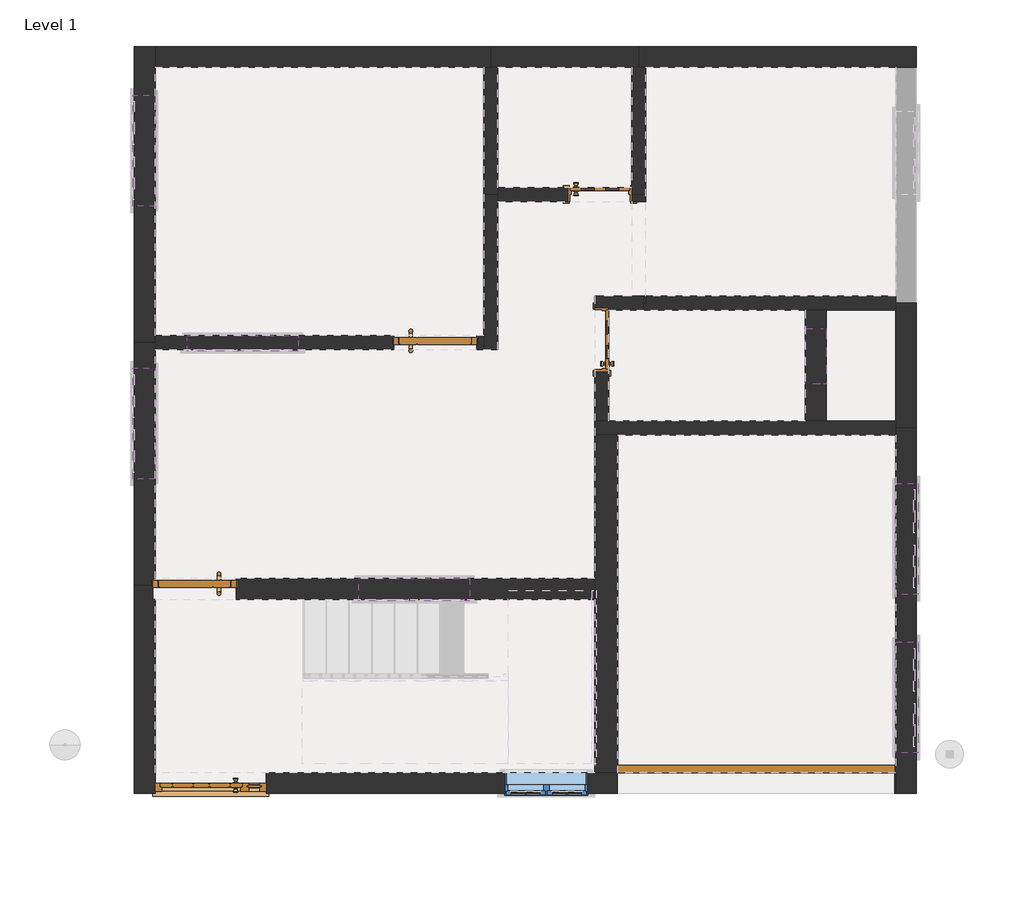
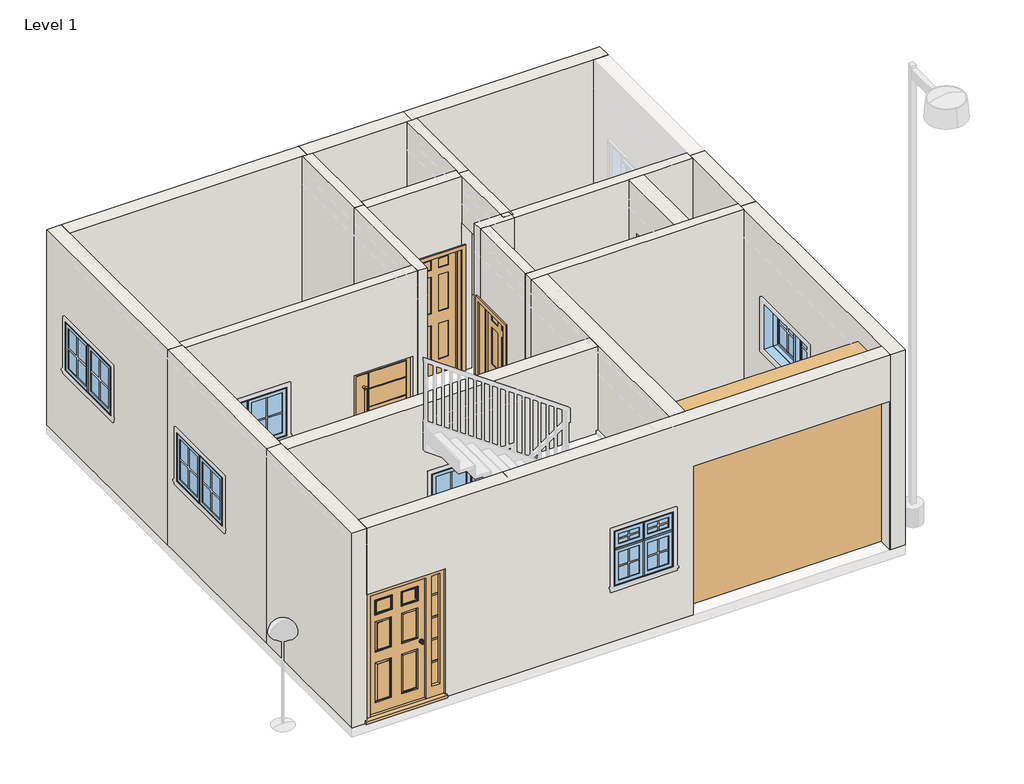
# One storey, part 1 of 3: 22 walls, 8 windows, 6 doors.
"""IFC4 building model written with IfcOpenShell, lengths in millimetres."""

from ifc_helpers import new_model, si_unit, frame, origin, place, context, project, spatial, polyline, outline, extrude, faceted_brep, transform, mapped, element, save
from components import door_3_ad1505b7, door_3_3562bf2b, extsgl_w_side_panel_4_ddded634, door_c4e61f94, door_c896847d, m_door_overhead_rolling_10_f67a646e, m_fixed_2_dd9f9b20, m_window_awning_double_horizontal_4_8afcb0b2, m_window_awning_double_horizontal_4_cab21571, m_window_casement_double_awning_double_3_6fa9dbfe

model = new_model("IFC4")

# Units and contexts
model_context = context("Model", 3, world=origin())
ifc_project = project(units=[si_unit("LENGTHUNIT", "METRE", prefix="MILLI")], contexts=[model_context])

# Site, building, storey
site = spatial("IfcSite", under=ifc_project)
building = spatial("IfcBuilding", under=site)
storey = spatial("IfcBuildingStorey", under=building, Name="Level 1", Elevation=0.0)

# Doors
placement = place(None, origin())
door_3_shape = door_3_ad1505b7(model_context)
element("IfcDoor", 1, ObjectType="3'", at=placement, inside=storey, context=model_context, shape_type="MappedRepresentation", body=[
    mapped(door_3_shape, transform((-8356.4282945, 391.3578397, 0.0), x_axis=(1.0, 0.0, 0.0), y_axis=(0.0, 1.0, 0.0), z_axis=(0.0, 0.0, 1.0))),
])
door_3_2_shape = door_3_3562bf2b(model_context)
element("IfcDoor", 2, ObjectType="3'", at=placement, inside=storey, context=model_context, shape_type="MappedRepresentation", body=[
    mapped(door_3_2_shape, transform((-10998.0282945, -2313.7421603, 0.0), x_axis=(-1.0, 0.0, 0.0), y_axis=(0.0, -1.0, 0.0), z_axis=(0.0, 0.0, 1.0))),
])
extsgl_w_side_panel_4_shape = extsgl_w_side_panel_4_ddded634(model_context)
element("IfcDoor", 3, ObjectType="ExtSgl w Side Panel : 4'", at=placement, inside=storey, context=model_context, shape_type="MappedRepresentation", body=[
    mapped(extsgl_w_side_panel_4_shape, transform((-11039.6282945, -4447.3421603, 0.0), x_axis=(-1.0, 0.0, 0.0), y_axis=(0.0, -1.0, 0.0), z_axis=(0.0, 0.0, 1.0))),
])
door_shape = door_c4e61f94(model_context)
element("IfcDoor", 4, ObjectType="M_Door-Interior-Single-6_Panel-Wood : 650 x 2000mm", at=placement, inside=storey, context=model_context, shape_type="MappedRepresentation", body=[
    mapped(door_shape, transform((-6547.4282945, 2020.1328397, 0.0), x_axis=(1.0, 0.0, 0.0), y_axis=(0.0, 1.0, 0.0), z_axis=(0.0, 0.0, 1.0))),
])
door_2_shape = door_c896847d(model_context)
element("IfcDoor", 5, ObjectType="M_Door-Interior-Single-6_Panel-Wood : 650 x 2000mm", at=placement, inside=storey, context=model_context, shape_type="MappedRepresentation", body=[
    mapped(door_2_shape, transform((-6524.4532945, 422.3578397, 0.0), x_axis=(0.0, 1.0, 0.0), y_axis=(-1.0, 0.0, 0.0), z_axis=(0.0, 0.0, 1.0))),
])
m_door_overhead_rolling_10_shape = m_door_overhead_rolling_10_f67a646e(model_context)
element("IfcDoor", 6, ObjectType="M_Door-Overhead-Rolling : 10'", at=placement, inside=storey, context=model_context, shape_type="MappedRepresentation", body=[
    mapped(m_door_overhead_rolling_10_shape, transform((-4834.0282945, -4447.3421603, 0.0289063), x_axis=(1.0, 0.0, 0.0), y_axis=(0.0, 1.0, 0.0), z_axis=(0.0, 0.0, 1.0))),
])

# Walls
element("IfcWall", 7, ObjectType="10\"", at=placement, inside=storey, context=model_context, shape_type="Brep", body=[
    faceted_brep([(-6603.8282945, -624.6421603, 0.0), (-6603.8282945, -2199.4421603, 0.0), (-6603.8282945, -2428.0421603, 0.0), (-6603.8282945, -4333.0421603, 0.0), (-6603.8282945, -4333.0421603, 3200.4), (-6603.8282945, -2428.0421603, 3200.4), (-6603.8282945, -2199.4421603, 3200.4), (-6603.8282945, -624.6421603, 3200.4), (-6349.8282945, -624.6421603, 0.0), (-6349.8282945, -624.6421603, 3200.4), (-6349.8282945, -4333.0421603, 3200.4), (-6349.8282945, -4333.0421603, 0.0)], [[[0, 1, 2, 3, 4, 5, 6, 7]], [[8, 9, 10, 11]], [[3, 2, 1, 0, 8, 11]], [[7, 6, 5, 4, 10, 9]], [[0, 7, 9, 8]], [[4, 3, 11, 10]]]),
])
element("IfcWall", 8, ObjectType="6\"", at=placement, inside=storey, context=model_context, shape_type="Brep", body=[
    faceted_brep([(-6197.4282945, 2016.9578397, 3200.4), (-6197.4282945, 2093.1578397, 3200.4), (-6197.4282945, 3413.9578397, 3200.4), (-6197.4282945, 3413.9578397, 0.0), (-6197.4282945, 2093.1578397, 0.0), (-6197.4282945, 2093.1578397, 2025.0), (-6197.4282945, 2016.9578397, 2025.0), (-6045.0282945, 2016.9578397, 0.0), (-6045.0282945, 3413.9578397, 0.0), (-6045.0282945, 3413.9578397, 3200.4), (-6045.0282945, 2016.9578397, 3200.4), (-6192.2282945, 2016.9578397, 0.0), (-6192.2282945, 2093.1578397, 0.0), (-6121.2282945, 3413.9578397, 0.0), (-6192.2282945, 2016.9578397, 2025.0), (-6121.2282945, 3413.9578397, 3200.4), (-6192.2282945, 2093.1578397, 2025.0)], [[[0, 1, 2, 3, 4, 5, 6]], [[7, 8, 9, 10]], [[8, 7, 11, 12, 4, 3, 13]], [[7, 10, 0, 6, 14, 11]], [[2, 1, 0, 10, 9, 15]], [[3, 2, 15, 9, 8, 13]], [[12, 16, 5, 4]], [[16, 12, 11, 14]], [[5, 16, 14, 6]]]),
])
element("IfcWall", 9, ObjectType="6\"", at=placement, inside=storey, context=model_context, shape_type="Brep", body=[
    faceted_brep([(-6070.4282945, 746.9578397, 0.0), (-6070.4282945, 746.9578397, 3200.4), (-6451.4282945, 746.9578397, 3200.4), (-6603.8282945, 746.9578397, 3200.4), (-6603.8282945, 746.9578397, 2025.0), (-6451.4282945, 746.9578397, 2025.0), (-6451.4282945, 746.9578397, 0.0), (-6070.4282945, 899.3578397, 0.0), (-6603.8282945, 899.3578397, 0.0), (-6603.8282945, 899.3578397, 3200.4), (-6070.4282945, 899.3578397, 3200.4), (-6451.4282945, 777.5578397, 0.0), (-6603.8282945, 777.5578397, 0.0), (-6603.8282945, 777.5578397, 2025.0), (-6451.4282945, 777.5578397, 2025.0)], [[[0, 1, 2, 3, 4, 5, 6]], [[7, 8, 9, 10]], [[8, 7, 0, 6, 11, 12]], [[1, 0, 7, 10]], [[3, 2, 1, 10, 9]], [[3, 9, 8, 12, 13, 4]], [[14, 11, 6, 5]], [[13, 14, 5, 4]], [[11, 14, 13, 12]]]),
])
element("IfcWall", 10, ObjectType="6\"", at=placement, inside=storey, context=model_context, shape_type="Brep", body=[
    faceted_brep([(-3301.8282945, -472.2421603, 0.0), (-4063.8282945, -472.2421603, 0.0), (-4292.4282945, -472.2421603, 0.0), (-6451.4282945, -472.2421603, 0.0), (-6603.8282945, -472.2421603, 0.0), (-6603.8282945, -472.2421603, 3200.4), (-6451.4282945, -472.2421603, 3200.4), (-4292.4282945, -472.2421603, 3200.4), (-4063.8282945, -472.2421603, 3200.4), (-3301.8282945, -472.2421603, 3200.4), (-3301.8282945, -624.6421603, 0.0), (-3301.8282945, -624.6421603, 3200.4), (-6349.8282945, -624.6421603, 3200.4), (-6603.8282945, -624.6421603, 3200.4), (-6603.8282945, -624.6421603, 0.0), (-6349.8282945, -624.6421603, 0.0), (-3301.8282945, -548.4421603, 0.0), (-3301.8282945, -548.4421603, 3200.4)], [[[0, 1, 2, 3, 4, 5, 6, 7, 8, 9]], [[10, 11, 12, 13, 14, 15]], [[4, 3, 2, 1, 0, 16, 10, 15, 14]], [[9, 8, 7, 6, 5, 13, 12, 11, 17]], [[0, 9, 17, 11, 10, 16]], [[5, 4, 14, 13]]]),
])
element("IfcWall", 11, ObjectType="6\"", at=placement, inside=storey, context=model_context, shape_type="Brep", body=[
    faceted_brep([(-7823.0282945, 3413.9578397, 0.0), (-7823.0282945, 2016.9578397, 0.0), (-7823.0282945, 2016.9578397, 3200.4), (-7823.0282945, 3413.9578397, 3200.4), (-7670.6282945, 3413.9578397, 0.0), (-7670.6282945, 3413.9578397, 3200.4), (-7670.6282945, 2093.1578397, 3200.4), (-7670.6282945, 2016.9578397, 3200.4), (-7670.6282945, 2016.9578397, 0.0), (-7670.6282945, 2093.1578397, 0.0), (-7746.8282945, 3413.9578397, 0.0), (-7746.8282945, 3413.9578397, 3200.4)], [[[0, 1, 2, 3]], [[4, 5, 6, 7, 8, 9]], [[1, 0, 10, 4, 9, 8]], [[2, 1, 8, 7]], [[3, 2, 7, 6, 5, 11]], [[0, 3, 11, 5, 4, 10]]]),
])
element("IfcWall", 12, ObjectType="6\"", at=placement, inside=storey, context=model_context, shape_type="Brep", body=[
    faceted_brep([(-7823.0282945, 315.1578397, 3200.4), (-11429.8282945, 315.1578397, 3200.4), (-11429.8282945, 315.1578397, 0.0), (-8813.6282945, 315.1578397, 0.0), (-8813.6282945, 315.1578397, 1828.8), (-7899.2282945, 315.1578397, 1828.8), (-7899.2282945, 315.1578397, 0.0), (-7823.0282945, 315.1578397, 0.0), (-11078.1970445, 315.1578397, 2019.2), (-9858.9970445, 315.1578397, 2019.2), (-9858.9970445, 315.1578397, 1219.2), (-11078.1970445, 315.1578397, 1219.2), (-11429.8282945, 467.5578397, 3200.4), (-7823.0282945, 467.5578397, 3200.4), (-7823.0282945, 467.5578397, 0.0), (-7899.2282945, 467.5578397, 0.0), (-7899.2282945, 467.5578397, 1828.8), (-8813.6282945, 467.5578397, 1828.8), (-8813.6282945, 467.5578397, 0.0), (-11429.8282945, 467.5578397, 0.0), (-11078.1970445, 467.5578397, 2019.2), (-11078.1970445, 467.5578397, 1219.2), (-9858.9970445, 467.5578397, 1219.2), (-9858.9970445, 467.5578397, 2019.2), (-11429.8282945, 391.3578397, 0.0), (-8813.6282945, 447.5578397, 0.0), (-8828.6282945, 447.5578397, 0.0), (-8828.6282945, 370.5578397, 0.0), (-8813.6282945, 370.5578397, 0.0), (-7899.2282945, 370.5578397, 0.0), (-7884.2282945, 370.5578397, 0.0), (-7884.2282945, 447.5578397, 0.0), (-7899.2282945, 447.5578397, 0.0), (-11429.8282945, 391.3578397, 3200.4), (-7899.2282945, 447.5578397, 1828.8), (-8813.6282945, 447.5578397, 1828.8), (-8813.6282945, 370.5578397, 1828.8), (-7899.2282945, 370.5578397, 1828.8), (-8828.6282945, 447.5578397, 1843.8), (-7884.2282945, 447.5578397, 1843.8), (-7884.2282945, 370.5578397, 1843.8), (-8828.6282945, 370.5578397, 1843.8)], [[[0, 1, 2, 3, 4, 5, 6, 7], [8, 9, 10, 11]], [[12, 13, 14, 15, 16, 17, 18, 19], [20, 21, 22, 23]], [[2, 24, 19, 18, 25, 26, 27, 28, 3]], [[14, 7, 6, 29, 30, 31, 32, 15]], [[1, 0, 13, 12, 33]], [[0, 7, 14, 13]], [[2, 1, 33, 12, 19, 24]], [[16, 34, 35, 17]], [[4, 36, 37, 5]], [[34, 16, 15, 32]], [[5, 37, 29, 6]], [[17, 35, 25, 18]], [[36, 4, 3, 28]], [[38, 39, 40, 41]], [[40, 39, 31, 30]], [[37, 36, 28, 27, 41, 40, 30, 29]], [[38, 41, 27, 26]], [[35, 34, 32, 31, 39, 38, 26, 25]], [[21, 20, 8, 11]], [[22, 21, 11, 10]], [[23, 22, 10, 9]], [[20, 23, 9, 8]]]),
])
element("IfcWall", 13, ObjectType="6\"", at=placement, inside=storey, context=model_context, shape_type="Brep", body=[
    faceted_brep([(-6197.4282945, 1940.7578397, 3200.4), (-7670.6282945, 1940.7578397, 3200.4), (-7670.6282945, 1940.7578397, 0.0), (-6902.6282945, 1940.7578397, 0.0), (-6902.6282945, 1940.7578397, 2025.0), (-6197.4282945, 1940.7578397, 2025.0), (-7670.6282945, 2093.1578397, 3200.4), (-6197.4282945, 2093.1578397, 3200.4), (-6197.4282945, 2093.1578397, 2025.0), (-6902.6282945, 2093.1578397, 2025.0), (-6902.6282945, 2093.1578397, 0.0), (-7670.6282945, 2093.1578397, 0.0), (-7670.6282945, 2016.9578397, 0.0), (-6197.4282945, 2016.9578397, 3200.4), (-7670.6282945, 2016.9578397, 3200.4), (-6197.4282945, 2016.9578397, 2025.0)], [[[0, 1, 2, 3, 4, 5]], [[6, 7, 8, 9, 10, 11]], [[2, 12, 11, 10, 3]], [[1, 0, 13, 7, 6, 14]], [[7, 13, 0, 5, 15, 8]], [[2, 1, 14, 6, 11, 12]], [[4, 9, 8, 15, 5]], [[9, 4, 3, 10]]]),
])
element("IfcWall", 14, ObjectType="6\"", at=placement, inside=storey, context=model_context, shape_type="SweptSolid", body=[
    extrude(outline(polyline([(-472.2421603, 3200.4), (746.9578397, 3200.4), (746.9578397, 2025.0), (67.1578397, 2025.0), (67.1578397, 0.0), (-472.2421603, 0.0), (-472.2421603, 3200.4)])), frame((-6603.8282945, 0.0, 0.0), z_axis=(1.0, 0.0, 0.0), x_axis=(0.0, 1.0, 0.0)), (0.0, 0.0, 1.0), 152.4),
])
element("IfcWall", 15, ObjectType="6\"", at=placement, inside=storey, context=model_context, shape_type="Brep", body=[
    faceted_brep([(-7823.0282945, 2016.9578397, 0.0), (-7823.0282945, 467.5578397, 0.0), (-7823.0282945, 315.1578397, 0.0), (-7823.0282945, 315.1578397, 3200.4), (-7823.0282945, 467.5578397, 3200.4), (-7823.0282945, 2016.9578397, 3200.4), (-7670.6282945, 2016.9578397, 0.0), (-7670.6282945, 2016.9578397, 3200.4), (-7670.6282945, 1940.7578397, 3200.4), (-7670.6282945, 315.1578397, 3200.4), (-7670.6282945, 315.1578397, 0.0), (-7670.6282945, 1940.7578397, 0.0)], [[[0, 1, 2, 3, 4, 5]], [[6, 7, 8, 9, 10, 11]], [[2, 1, 0, 6, 11, 10]], [[5, 4, 3, 9, 8, 7]], [[0, 5, 7, 6]], [[3, 2, 10, 9]]]),
])
element("IfcWall", 16, ObjectType="6\"", at=placement, inside=storey, context=model_context, shape_type="Brep", body=[
    faceted_brep([(-6197.4282945, 823.1578397, 0.0), (-6197.4282945, 823.1578397, 3200.4), (-6197.4282945, 1940.7578397, 3200.4), (-6197.4282945, 2016.9578397, 3200.4), (-6197.4282945, 2016.9578397, 2025.0), (-6197.4282945, 1940.7578397, 2025.0), (-6197.4282945, 1940.7578397, 0.0), (-6197.4282945, 1939.2741832, 0.0), (-6197.4282945, 1939.2741832, 2438.4), (-6197.4282945, 896.0499365, 2438.4), (-6197.4282945, 896.0499365, 0.0), (-6045.0282945, 823.1578397, 3200.4), (-6045.0282945, 823.1578397, 0.0), (-6045.0282945, 896.0499365, 0.0), (-6045.0282945, 896.0499365, 2438.4), (-6045.0282945, 1939.2741832, 2438.4), (-6045.0282945, 1939.2741832, 0.0), (-6045.0282945, 2016.9578397, 0.0), (-6045.0282945, 2016.9578397, 3200.4), (-6192.2282945, 1940.7578397, 0.0), (-6192.2282945, 2016.9578397, 0.0), (-6192.2282945, 2016.9578397, 2025.0), (-6192.2282945, 1940.7578397, 2025.0)], [[[0, 1, 2, 3, 4, 5, 6, 7, 8, 9, 10]], [[11, 12, 13, 14, 15, 16, 17, 18]], [[12, 0, 10, 13]], [[17, 16, 7, 6, 19, 20]], [[1, 0, 12, 11]], [[3, 2, 1, 11, 18]], [[18, 17, 20, 21, 4, 3]], [[8, 15, 14, 9]], [[15, 8, 7, 16]], [[9, 14, 13, 10]], [[22, 19, 6, 5]], [[19, 22, 21, 20]], [[22, 5, 4, 21]]]),
])
element("IfcWall", 17, ObjectType="6\"", at=placement, inside=storey, context=model_context, shape_type="Brep", body=[
    faceted_brep([(-6070.4282945, 746.9578397, 0.0), (-4292.4282945, 746.9578397, 0.0), (-4063.8282945, 746.9578397, 0.0), (-3301.8282945, 746.9578397, 0.0), (-3301.8282945, 746.9578397, 3200.4), (-4063.8282945, 746.9578397, 3200.4), (-4292.4282945, 746.9578397, 3200.4), (-6070.4282945, 746.9578397, 3200.4), (-6070.4282945, 899.3578397, 0.0), (-6070.4282945, 899.3578397, 3200.4), (-3301.8282945, 899.3578397, 3200.4), (-3301.8282945, 899.3578397, 0.0), (-3301.8282945, 823.1578397, 0.0), (-3301.8282945, 823.1578397, 3200.4)], [[[0, 1, 2, 3, 4, 5, 6, 7]], [[8, 9, 10, 11]], [[3, 2, 1, 0, 8, 11, 12]], [[7, 6, 5, 4, 13, 10, 9]], [[0, 7, 9, 8]], [[4, 3, 12, 11, 10, 13]]]),
])
element("IfcWall", 18, ObjectType="9\"", at=placement, inside=storey, context=model_context, shape_type="Brep", body=[
    faceted_brep([(-11658.4282945, 3642.5578397, 0.0), (-11658.4282945, 391.3578397, 0.0), (-11658.4282945, 391.3578397, 3200.4), (-11658.4282945, 3642.5578397, 3200.4), (-11658.4282945, 3109.1578397, 2019.2), (-11658.4282945, 1889.9578397, 2019.2), (-11658.4282945, 1889.9578397, 1219.2), (-11658.4282945, 3109.1578397, 1219.2), (-11429.8282945, 3642.5578397, 0.0), (-11429.8282945, 3642.5578397, 3200.4), (-11429.8282945, 3413.9578397, 3200.4), (-11429.8282945, 467.5578397, 3200.4), (-11429.8282945, 391.3578397, 3200.4), (-11429.8282945, 391.3578397, 0.0), (-11429.8282945, 467.5578397, 0.0), (-11429.8282945, 3413.9578397, 0.0), (-11429.8282945, 3109.1578397, 2019.2), (-11429.8282945, 3109.1578397, 1219.2), (-11429.8282945, 1889.9578397, 1219.2), (-11429.8282945, 1889.9578397, 2019.2)], [[[0, 1, 2, 3], [4, 5, 6, 7]], [[8, 9, 10, 11, 12, 13, 14, 15], [16, 17, 18, 19]], [[1, 0, 8, 15, 14, 13]], [[2, 1, 13, 12]], [[3, 2, 12, 11, 10, 9]], [[0, 3, 9, 8]], [[17, 16, 4, 7]], [[18, 17, 7, 6]], [[19, 18, 6, 5]], [[16, 19, 5, 4]]]),
])
element("IfcWall", 19, ObjectType="9\"", at=placement, inside=storey, context=model_context, shape_type="Brep", body=[
    faceted_brep([(-11429.8282945, 3413.9578397, 0.0), (-7823.0282945, 3413.9578397, 0.0), (-7746.8282945, 3413.9578397, 0.0), (-7746.8282945, 3413.9578397, 3200.4), (-7823.0282945, 3413.9578397, 3200.4), (-11429.8282945, 3413.9578397, 3200.4), (-11429.8282945, 3642.5578397, 0.0), (-11429.8282945, 3642.5578397, 3200.4), (-7746.8282945, 3642.5578397, 3200.4), (-7746.8282945, 3642.5578397, 0.0)], [[[0, 1, 2, 3, 4, 5]], [[6, 7, 8, 9]], [[2, 1, 0, 6, 9]], [[3, 2, 9, 8]], [[5, 4, 3, 8, 7]], [[0, 5, 7, 6]]]),
])
element("IfcWall", 20, ObjectType="9\"", at=placement, inside=storey, context=model_context, shape_type="Brep", body=[
    faceted_brep([(-11429.8282945, -4333.0421603, 3200.4), (-6603.8282945, -4333.0421603, 3200.4), (-6349.8282945, -4333.0421603, 3200.4), (-3301.8282945, -4333.0421603, 3200.4), (-3301.8282945, -4333.0421603, 0.0), (-3310.0282945, -4333.0421603, 0.0), (-3310.0282945, -4333.0421603, 2438.4289062), (-6358.0282945, -4333.0421603, 2438.4289062), (-6358.0282945, -4333.0421603, 0.0), (-6603.8282945, -4333.0421603, 0.0), (-10210.6282945, -4333.0421603, 0.0), (-10210.6282945, -4333.0421603, 2110.0), (-11429.8282945, -4333.0421603, 2110.0), (-7594.4282945, -4333.0421603, 1814.4), (-7594.4282945, -4333.0421603, 914.4), (-6680.0282945, -4333.0421603, 914.4), (-6680.0282945, -4333.0421603, 1814.4), (-3301.8282945, -4561.6421603, 3200.4), (-11429.8282945, -4561.6421603, 3200.4), (-11429.8282945, -4561.6421603, 2110.0), (-10210.6282945, -4561.6421603, 2110.0), (-10210.6282945, -4561.6421603, 0.0), (-6358.0282945, -4561.6421603, 0.0), (-6358.0282945, -4561.6421603, 2438.4289062), (-3310.0282945, -4561.6421603, 2438.4289062), (-3310.0282945, -4561.6421603, 0.0), (-3301.8282945, -4561.6421603, 0.0), (-7594.4282945, -4561.6421603, 1814.4), (-6680.0282945, -4561.6421603, 1814.4), (-6680.0282945, -4561.6421603, 914.4), (-7594.4282945, -4561.6421603, 914.4)], [[[0, 1, 2, 3, 4, 5, 6, 7, 8, 9, 10, 11, 12], [13, 14, 15, 16]], [[17, 18, 19, 20, 21, 22, 23, 24, 25, 26], [27, 28, 29, 30]], [[4, 26, 25, 5]], [[8, 22, 21, 10, 9]], [[3, 2, 1, 0, 18, 17]], [[18, 0, 12, 19]], [[4, 3, 17, 26]], [[6, 5, 25, 24]], [[7, 6, 24, 23]], [[8, 7, 23, 22]], [[20, 11, 10, 21]], [[11, 20, 19, 12]], [[14, 13, 27, 30]], [[15, 14, 30, 29]], [[16, 15, 29, 28]], [[13, 16, 28, 27]]]),
])
element("IfcWall", 21, ObjectType="9\"", at=placement, inside=storey, context=model_context, shape_type="Brep", body=[
    faceted_brep([(-11429.8282945, -2199.4421603, 3200.4), (-6603.8282945, -2199.4421603, 3200.4), (-6603.8282945, -2199.4421603, 0.0), (-10540.8282945, -2199.4421603, 0.0), (-10540.8282945, -2199.4421603, 1828.8), (-11429.8282945, -2199.4421603, 1828.8), (-9194.6282945, -2199.4421603, 2019.2), (-9194.6282945, -2199.4421603, 1219.2), (-7975.4282945, -2199.4421603, 1219.2), (-7975.4282945, -2199.4421603, 2019.2), (-6603.8282945, -2428.0421603, 3200.4), (-11429.8282945, -2428.0421603, 3200.4), (-11429.8282945, -2428.0421603, 1828.8), (-10540.8282945, -2428.0421603, 1828.8), (-10540.8282945, -2428.0421603, 0.0), (-6603.8282945, -2428.0421603, 0.0), (-9194.6282945, -2428.0421603, 2019.2), (-7975.4282945, -2428.0421603, 2019.2), (-7975.4282945, -2428.0421603, 1219.2), (-9194.6282945, -2428.0421603, 1219.2), (-10540.8282945, -2296.4421603, 0.0), (-10525.8282945, -2296.4421603, 0.0), (-10525.8282945, -2219.4421603, 0.0), (-10540.8282945, -2219.4421603, 0.0), (-11429.8282945, -2275.6421603, 3200.4), (-11429.8282945, -2219.4421603, 1828.8), (-11429.8282945, -2219.4421603, 1843.8), (-11429.8282945, -2296.4421603, 1843.8), (-11429.8282945, -2296.4421603, 1828.8), (-10540.8282945, -2219.4421603, 1828.8), (-10540.8282945, -2296.4421603, 1828.8), (-10525.8282945, -2219.4421603, 1843.8), (-10525.8282945, -2296.4421603, 1843.8)], [[[0, 1, 2, 3, 4, 5], [6, 7, 8, 9]], [[10, 11, 12, 13, 14, 15], [16, 17, 18, 19]], [[2, 15, 14, 20, 21, 22, 23, 3]], [[1, 0, 24, 11, 10]], [[11, 24, 0, 5, 25, 26, 27, 28, 12]], [[2, 1, 10, 15]], [[4, 29, 25, 5]], [[30, 13, 12, 28]], [[29, 4, 3, 23]], [[13, 30, 20, 14]], [[31, 32, 27, 26]], [[20, 30, 28, 27, 32, 21]], [[32, 31, 22, 21]], [[29, 23, 22, 31, 26, 25]], [[7, 6, 16, 19]], [[8, 7, 19, 18]], [[9, 8, 18, 17]], [[6, 9, 17, 16]]]),
])
element("IfcWall", 22, ObjectType="9\"", at=placement, inside=storey, context=model_context, shape_type="SweptSolid", body=[
    extrude(outline(polyline([(746.9578397, 0.0), (-472.2421603, 0.0), (-472.2421603, 3200.4), (746.9578397, 3200.4), (746.9578397, 0.0)]), holes=[polyline([(543.7578397, 2133.6), (543.7578397, 2438.4), (-65.8421603, 2438.4), (-65.8421603, 2133.6), (543.7578397, 2133.6)])]), frame((-4292.4282945, 0.0, 0.0), z_axis=(1.0, 0.0, 0.0), x_axis=(0.0, 1.0, 0.0)), (0.0, 0.0, 1.0), 228.6),
])
element("IfcWall", 23, ObjectType="9\"", at=placement, inside=storey, context=model_context, shape_type="Brep", body=[
    faceted_brep([(-11658.4282945, 391.3578397, 0.0), (-11658.4282945, -2275.6421603, 0.0), (-11658.4282945, -2275.6421603, 3200.4), (-11658.4282945, 391.3578397, 3200.4), (-11658.4282945, 111.9578397, 2019.2), (-11658.4282945, -1107.2421603, 2019.2), (-11658.4282945, -1107.2421603, 1219.2), (-11658.4282945, 111.9578397, 1219.2), (-11429.8282945, 391.3578397, 3200.4), (-11429.8282945, 315.1578397, 3200.4), (-11429.8282945, -2275.6421603, 3200.4), (-11429.8282945, -2275.6421603, 1843.8), (-11429.8282945, -2219.4421603, 1843.8), (-11429.8282945, -2219.4421603, 1828.8), (-11429.8282945, -2199.4421603, 1828.8), (-11429.8282945, -2199.4421603, 0.0), (-11429.8282945, 315.1578397, 0.0), (-11429.8282945, 391.3578397, 0.0), (-11429.8282945, 111.9578397, 2019.2), (-11429.8282945, 111.9578397, 1219.2), (-11429.8282945, -1107.2421603, 1219.2), (-11429.8282945, -1107.2421603, 2019.2), (-11455.2282945, -2199.4421603, 0.0), (-11455.2282945, -2219.4421603, 0.0), (-11470.2282945, -2219.4421603, 0.0), (-11470.2282945, -2275.6421603, 0.0), (-11470.2282945, -2275.6421603, 1843.8), (-11455.2282945, -2199.4421603, 1828.8), (-11455.2282945, -2219.4421603, 1828.8), (-11470.2282945, -2219.4421603, 1843.8)], [[[0, 1, 2, 3], [4, 5, 6, 7]], [[8, 9, 10, 11, 12, 13, 14, 15, 16, 17], [18, 19, 20, 21]], [[1, 0, 17, 16, 15, 22, 23, 24, 25]], [[2, 1, 25, 26, 11, 10]], [[3, 2, 10, 9, 8]], [[0, 3, 8, 17]], [[18, 21, 5, 4]], [[21, 20, 6, 5]], [[20, 19, 7, 6]], [[19, 18, 4, 7]], [[27, 22, 15, 14]], [[28, 27, 14, 13]], [[22, 27, 28, 23]], [[26, 29, 12, 11]], [[24, 29, 26, 25]], [[23, 28, 13, 12, 29, 24]]]),
])
element("IfcWall", 24, ObjectType="9\"", at=placement, inside=storey, context=model_context, shape_type="Brep", body=[
    faceted_brep([(-7746.8282945, 3413.9578397, 0.0), (-7670.6282945, 3413.9578397, 0.0), (-6197.4282945, 3413.9578397, 0.0), (-6121.2282945, 3413.9578397, 0.0), (-6121.2282945, 3413.9578397, 3200.4), (-6197.4282945, 3413.9578397, 3200.4), (-7670.6282945, 3413.9578397, 3200.4), (-7746.8282945, 3413.9578397, 3200.4), (-7746.8282945, 3642.5578397, 0.0), (-7746.8282945, 3642.5578397, 3200.4), (-6121.2282945, 3642.5578397, 3200.4), (-6121.2282945, 3642.5578397, 0.0)], [[[0, 1, 2, 3, 4, 5, 6, 7]], [[8, 9, 10, 11]], [[3, 2, 1, 0, 8, 11]], [[4, 3, 11, 10]], [[7, 6, 5, 4, 10, 9]], [[0, 7, 9, 8]]]),
])
element("IfcWall", 25, ObjectType="9\"", at=placement, inside=storey, context=model_context, shape_type="Brep", body=[
    faceted_brep([(-6121.2282945, 3413.9578397, 0.0), (-6045.0282945, 3413.9578397, 0.0), (-3301.8282945, 3413.9578397, 0.0), (-3073.2282945, 3413.9578397, 0.0), (-3073.2282945, 3413.9578397, 3200.4), (-3301.8282945, 3413.9578397, 3200.4), (-6045.0282945, 3413.9578397, 3200.4), (-6121.2282945, 3413.9578397, 3200.4), (-6121.2282945, 3642.5578397, 0.0), (-6121.2282945, 3642.5578397, 3200.4), (-3073.2282945, 3642.5578397, 3200.4), (-3073.2282945, 3642.5578397, 0.0)], [[[0, 1, 2, 3, 4, 5, 6, 7]], [[8, 9, 10, 11]], [[3, 2, 1, 0, 8, 11]], [[7, 6, 5, 4, 10, 9]], [[0, 7, 9, 8]], [[4, 3, 11, 10]]]),
])
element("IfcWall", 26, ObjectType="9\"", at=placement, inside=storey, context=model_context, shape_type="Brep", body=[
    faceted_brep([(-3301.8282945, 823.1578397, 0.0), (-3301.8282945, 746.9578397, 0.0), (-3301.8282945, -472.2421603, 0.0), (-3301.8282945, -548.4421603, 0.0), (-3301.8282945, -548.4421603, 3200.4), (-3301.8282945, -472.2421603, 3200.4), (-3301.8282945, 746.9578397, 3200.4), (-3301.8282945, 823.1578397, 3200.4), (-3073.2282945, 823.1578397, 0.0), (-3073.2282945, 823.1578397, 3200.4), (-3073.2282945, -548.4421603, 3200.4), (-3073.2282945, -548.4421603, 0.0)], [[[0, 1, 2, 3, 4, 5, 6, 7]], [[8, 9, 10, 11]], [[3, 2, 1, 0, 8, 11]], [[4, 3, 11, 10]], [[7, 6, 5, 4, 10, 9]], [[0, 7, 9, 8]]]),
])
element("IfcWall", 27, ObjectType="9\"", at=placement, inside=storey, context=model_context, shape_type="Brep", body=[
    faceted_brep([(-3301.8282945, -548.4421603, 0.0), (-3301.8282945, -624.6421603, 0.0), (-3301.8282945, -4333.0421603, 0.0), (-3301.8282945, -4561.6421603, 0.0), (-3301.8282945, -4561.6421603, 3200.4), (-3301.8282945, -4333.0421603, 3200.4), (-3301.8282945, -624.6421603, 3200.4), (-3301.8282945, -548.4421603, 3200.4), (-3301.8282945, -4117.1421603, 2019.2), (-3301.8282945, -4117.1421603, 1219.2), (-3301.8282945, -2897.9421603, 1219.2), (-3301.8282945, -2897.9421603, 2019.2), (-3301.8282945, -2374.4640353, 2019.2), (-3301.8282945, -2374.4640353, 1219.2), (-3301.8282945, -1155.2640353, 1219.2), (-3301.8282945, -1155.2640353, 2019.2), (-3073.2282945, -548.4421603, 0.0), (-3073.2282945, -548.4421603, 3200.4), (-3073.2282945, -4561.6421603, 3200.4), (-3073.2282945, -4561.6421603, 0.0), (-3073.2282945, -4117.1421603, 2019.2), (-3073.2282945, -2897.9421603, 2019.2), (-3073.2282945, -2897.9421603, 1219.2), (-3073.2282945, -4117.1421603, 1219.2), (-3073.2282945, -2374.4640353, 2019.2), (-3073.2282945, -1155.2640353, 2019.2), (-3073.2282945, -1155.2640353, 1219.2), (-3073.2282945, -2374.4640353, 1219.2)], [[[0, 1, 2, 3, 4, 5, 6, 7], [8, 9, 10, 11], [12, 13, 14, 15]], [[16, 17, 18, 19], [20, 21, 22, 23], [24, 25, 26, 27]], [[3, 2, 1, 0, 16, 19]], [[7, 6, 5, 4, 18, 17]], [[0, 7, 17, 16]], [[4, 3, 19, 18]], [[8, 11, 21, 20]], [[11, 10, 22, 21]], [[10, 9, 23, 22]], [[9, 8, 20, 23]], [[12, 15, 25, 24]], [[15, 14, 26, 25]], [[14, 13, 27, 26]], [[13, 12, 24, 27]]]),
])
element("IfcWall", 28, ObjectType="9\"", at=placement, inside=storey, context=model_context, shape_type="Brep", body=[
    faceted_brep([(-11658.4282945, -2275.6421603, 0.0), (-11658.4282945, -4561.6421603, 0.0), (-11658.4282945, -4561.6421603, 3200.4), (-11658.4282945, -2275.6421603, 3200.4), (-11429.8282945, -2275.6421603, 3200.4), (-11429.8282945, -2428.0421603, 3200.4), (-11429.8282945, -4333.0421603, 3200.4), (-11429.8282945, -4561.6421603, 3200.4), (-11429.8282945, -4561.6421603, 2110.0), (-11429.8282945, -4561.6421603, 0.0), (-11429.8282945, -2428.0421603, 0.0), (-11429.8282945, -2428.0421603, 1828.8), (-11429.8282945, -2296.4421603, 1828.8), (-11429.8282945, -2296.4421603, 1843.8), (-11429.8282945, -2275.6421603, 1843.8), (-11470.2282945, -2275.6421603, 0.0), (-11470.2282945, -2296.4421603, 0.0), (-11455.2282945, -2296.4421603, 0.0), (-11455.2282945, -2428.0421603, 0.0), (-11470.2282945, -2275.6421603, 1843.8), (-11455.2282945, -2428.0421603, 1828.8), (-11455.2282945, -2296.4421603, 1828.8), (-11470.2282945, -2296.4421603, 1843.8)], [[[0, 1, 2, 3]], [[4, 5, 6, 7, 8, 9, 10, 11, 12, 13, 14]], [[1, 0, 15, 16, 17, 18, 10, 9]], [[3, 2, 7, 6, 5, 4]], [[0, 3, 4, 14, 19, 15]], [[2, 1, 9, 8, 7]], [[18, 20, 11, 10]], [[20, 21, 12, 11]], [[20, 18, 17, 21]], [[13, 22, 19, 14]], [[22, 16, 15, 19]], [[21, 17, 16, 22, 13, 12]]]),
])

# Windows
m_fixed_2_shape = m_fixed_2_dd9f9b20(model_context)
element("IfcWindow", 29, ObjectType="M_Fixed : 2'", at=placement, inside=storey, context=model_context, shape_type="MappedRepresentation", body=[
    mapped(m_fixed_2_shape, transform((-4191.1282945, 238.9578397, 1218.6), x_axis=(0.0, -1.0, 0.0), y_axis=(1.0, 0.0, 0.0), z_axis=(0.0, 0.0, 1.0))),
])
m_window_awning_double_horizontal_4_shape = m_window_awning_double_horizontal_4_8afcb0b2(model_context)
element("IfcWindow", 30, ObjectType="M_Window-Awning-Double-Horizontal : 4'", at=placement, inside=storey, context=model_context, shape_type="MappedRepresentation", body=[
    mapped(m_window_awning_double_horizontal_4_shape, transform((-8585.0282945, -2313.7421603, 319.2), x_axis=(-1.0, 0.0, 0.0), y_axis=(0.0, -1.0, 0.0), z_axis=(0.0, 0.0, 1.0))),
])
element("IfcWindow", 31, ObjectType="M_Window-Awning-Double-Horizontal : 4'", at=placement, inside=storey, context=model_context, shape_type="MappedRepresentation", body=[
    mapped(m_window_awning_double_horizontal_4_shape, transform((-3187.5282945, -3507.5421603, 319.2), x_axis=(0.0, -1.0, 0.0), y_axis=(1.0, 0.0, 0.0), z_axis=(0.0, 0.0, 1.0))),
])
element("IfcWindow", 32, ObjectType="M_Window-Awning-Double-Horizontal : 4'", at=placement, inside=storey, context=model_context, shape_type="MappedRepresentation", body=[
    mapped(m_window_awning_double_horizontal_4_shape, transform((-3187.5282945, -1764.8640353, 319.2), x_axis=(0.0, -1.0, 0.0), y_axis=(1.0, 0.0, 0.0), z_axis=(0.0, 0.0, 1.0))),
])
element("IfcWindow", 33, ObjectType="M_Window-Awning-Double-Horizontal : 4'", at=placement, inside=storey, context=model_context, shape_type="MappedRepresentation", body=[
    mapped(m_window_awning_double_horizontal_4_shape, transform((-11544.1282945, 2499.5578397, 319.2), x_axis=(0.0, 1.0, 0.0), y_axis=(-1.0, 0.0, 0.0), z_axis=(0.0, 0.0, 1.0))),
])
element("IfcWindow", 34, ObjectType="M_Window-Awning-Double-Horizontal : 4'", at=placement, inside=storey, context=model_context, shape_type="MappedRepresentation", body=[
    mapped(m_window_awning_double_horizontal_4_shape, transform((-11544.1282945, -497.6421603, 319.2), x_axis=(0.0, 1.0, 0.0), y_axis=(-1.0, 0.0, 0.0), z_axis=(0.0, 0.0, 1.0))),
])
m_window_awning_double_horizontal_4_2_shape = m_window_awning_double_horizontal_4_cab21571(model_context)
element("IfcWindow", 35, ObjectType="M_Window-Awning-Double-Horizontal : 4'", at=placement, inside=storey, context=model_context, shape_type="MappedRepresentation", body=[
    mapped(m_window_awning_double_horizontal_4_2_shape, transform((-10468.5970445, 391.3578397, 319.2), x_axis=(-1.0, 0.0, 0.0), y_axis=(0.0, -1.0, 0.0), z_axis=(0.0, 0.0, 1.0))),
])
m_window_casement_double_awning_double_3_shape = m_window_casement_double_awning_double_3_6fa9dbfe(model_context)
element("IfcWindow", 36, ObjectType="M_Window-Casement-Double-Awning-Double : 3'", at=placement, inside=storey, context=model_context, shape_type="MappedRepresentation", body=[
    mapped(m_window_casement_double_awning_double_3_shape, transform((-7137.2282945, -4447.3421603, 14.4), x_axis=(-1.0, 0.0, 0.0), y_axis=(0.0, -1.0, 0.0), z_axis=(0.0, 0.0, 1.0))),
])

save(model, "model.ifc")

# Revit data of these elements
# Type "3'"
#   Type Mark = "41"
#   Water resistance = "up to Class E900, EN 12208:2001"
#   Uniclass2015Version = "v1.21"
#   Uniclass2015Reference = "Ss_25_30_20_30"
#   Uniclass2015Description = "Frame and door leaf system"
#   URL = "www.aluprof.com"
#   Type IFC Predefined Type = "USERDEFINED"
#   Right-hand / Left-hand door [instance default] = ""
#   Resistance to wind load = "up to Class C5/B5, EN 12210:2001"
#   Insert type = "ST"
#   Hardware [instance default] = ""
#   Product page = "https://aluprof.com/en/architects/offer/window-and-door-systems/panel-doors#visualisation"
#   Operation = "SinglePanelOutwardOpening"
#   Opening type = "Outward"
#   NBSReference = "25-50-20/125"
#   NBSDescription = "Frame and door leaf system"
#   Important = "The actual acceptable construction dimensions are dependent on the selection of profiles and hardware, glazing type, construction weight and the construction’s operating conditions. These should be determined by a suitably qualified person, and using ALUPROF’s calculation software"
#   IfcExportType = "USERDEFINED"
#   IfcExportAs = "IfcDoorType"
#   Handle type [instance default] = ""
#   Manufacturer = "ALUPROF SA"
#   Export Type to IFC As = "IfcDoorType"
#   Door sill type [instance default] = ""
#   Description = "External single-leaf panel door outward opening"
#   Model = "MB-86 ST Panel Door AD07"
#   Content of the recyclate in the material = "69.2%"
#   COBie.Type.WarrantyDurationParts = ""
#   COBie.Type.Name = ""
#   COBie.Type.Manufacturer = "ALUPROF SA"
#   COBie.Space.Name = ""
#   COBie.Floor.Name = ""
#   COBie.Facility.Name = ""
#   COBie.CreatedOn = ""
#   COBie.Component.WarrantyStartDate = ""
#   COBie.Component.Name = "MB-86 ST Panel Door AD07"
#   Burglar resistance = "RC2"
#   Air permeability = "up to Class 4, EN 12207:2001"
#   Width of the active leaf = 2' - 8.17717"
#   Placement in wall = 0' - 0.7874"
#   Thickness = 0' - 3.0315"
#   Height of the opening sash = 5' - 9.44094"
#   Handle Offset = 3' - 5.33858"
#   Rough Height = 6' - 2.40945"
#   Rough Width = 3' - 1.1811"
#   Height = 6' - 0"
#   Width = 3' - 0"
#   Construction depth = 0' - 3.0315"
#   Clear opening width = 2' - 3.94882"
#   Clear opening height = 5' - 8.47638"
#   Height of the array = 0' - 11.08136"
#   Schedule No. [instance default] = 1
#   Handrail [instance default] = yes
#   IsExternal = yes
#   Handle [instance default] = no
#   Door closer [instance default] = no
#   Function = 1
#   COBie.Type = yes
#   COBie = yes
#   Access control [instance default] = no
#   Panel = element 371215
#   Wall Closure = (empty or 0)
# Type "ExtSgl w Side Panel : 4'"
#   Type Mark = "46"
#   Operation = "SingleSwingRight"
#   Keynote = "L20"
#   Wrap Layers (Int) from Ext = 0' - 6.98819"
#   Wrap Layers (Ext) from Ext = 0' - 4.03543"
#   Thickness = 0' - 1.73228"
#   Stile Top of Lock rail = 3' - 3.37008"
#   Stile Top of Frieze Rail = 5' - 3.97638"
#   Stile Top Rail = 0' - 5.90551"
#   Stile Shutting = 0' - 4.92126"
#   Panelling Widths = 0' - 9.84252"
#   Stile Lock Rail = 0' - 6.88976"
#   Stile Intermediate/Frieze = 0' - 4.92126"
#   Stile Hanging = 0' - 4.92126"
#   Stile Bottom Rail = 0' - 6.88976"
#   Rough Width = 4' - 0"
#   Rough Height = 6' - 11.07087"
#   O/A Frame Width = 0' - 2.51969"
#   Handle Z Distance = 3' - 3.37008"
#   Glazing Thickness = 0' - 0.94488"
#   Glazing Bar Thickness = 0' - 0.98425"
#   FrameWidth = 0' - 1.65354"
#   FrameOffset - External = 0' - 0.98425"
#   FrameDepth = 0' - 3.50394"
#   Door Panel Width = 2' - 11.70866"
#   Door Panel Thickness = 0' - 1.73228"
#   Door Panel Height = 6' - 6.74016"
#   Cill Thickness = 0' - 2.14567"
#   Cill Projection = 0' - 1.1811"
#   Handle X Distance = 0' - 2.95276"
#   Height = 6' - 11.07087"
#   Structural Tolerance = 0' - 0.25591"
#   Tolerance = 0' - 0.11811"
#   Undercut = 0' - 0.15748"
#   Width = 4' - 0"
#   Cill Extension = 0' - 0.98425"
#   Cavity Closer Width = 0' - 1.9685"
#   Cavity Closer Offset from Ext = 0' - 4.03543"
#   Cavity Closer Depth = 0' - 3.34646"
#   Vis - SideLight Glazing Bars = yes
#   Vis - Ironmongery = yes
#   Vis - Cavity Closers = yes
#   Function = 1
#   Material Glass = Door - Glazing
#   Handle Style = element 379092
#   Material Door = Door - Panel
#   Material Ironmongery = Door - Handle
#   Wall Closure = (empty or 0)
# Type "M_Door-Interior-Single-6_Panel-Wood : 650 x 2000mm"
#   Type Mark = "42"
#   Assembly Code = "C1020300"
#   Analytic Construction = "Wooden"
#   Top Rail = 0' - 4.72441"
#   Top Panel = 0' - 6.01181"
#   Thickness = 0' - 1.37795"
#   Thermal Resistance (R) = 0.455703 (m²·K)/W
#   Swing Angle [instance default] = 90.00°
#   Stiles = 0' - 4.72441"
#   Rough Width = 2' - 3.9685"
#   Rough Height = 6' - 7.72441"
#   Mullion = 0' - 4.52756"
#   Lock Rail = 0' - 7.87402"
#   Intermediate Rail = 0' - 4.52756"
#   Height = 6' - 6.74016"
#   Width = 2' - 2"
#   Heat Transfer Coefficient (U) = 2.19465 W/(m²·K)
#   Bottom Rail = 0' - 9.05512"
#   Trim Material = Cherry
#   Panel Material = Cherry
#   Frame Material = Cherry
#   Door Handle Material = Aluminum
#   Visual Light Transmittance = 0
#   Solar Heat Gain Coefficient = 0
#   Wall Closure = (empty or 0)
#   Function = (empty or 0)
# Type "M_Door-Overhead-Rolling : 10'"
#   Type Mark = "44"
#   Construction Type Id = "MDOOR"
#   Assembly Code = "B2030400"
#   Analytic Construction = "Metal"
#   Thickness = 0' - 3.14961"
#   Rough Width [instance default] = 13' - 9.35433"
#   Rough Height [instance default] = 13' - 9.35433"
#   Heat Transfer Coefficient (U) = 3.7021 W/(m²·K)
#   Height [instance default] = 13' - 9.35433"
#   Width [instance default] = 13' - 9.35433"
#   Define Thermal Properties by = 1
#   Function = 1
#   Roller Material = Steel, Paint Finish, Ivory, Matte
#   Roller Box Material = Steel, Paint Finish, Ivory, Matte
#   Visual Light Transmittance = 0
#   Solar Heat Gain Coefficient = 0
#   Wall Closure = (empty or 0)
# Type "10\""
#   Layers, outside or top first: 0' - 10" no material (function 1)
# Type "6\""
#   Layers, outside or top first: 0' - 6" no material (function 1)
# Type "9\""
#   Layers, outside or top first: 0' - 9" no material (function 1)
# Type "M_Fixed : 2'"
#   Type Mark = "32"
#   Construction Type Id = "GSP4R"
#   Analytic Construction = "1/8 in Pilkington single glazing"
#   Visual Light Transmittance = 0.9
#   Thermal Resistance (R) = 0.271106 (m²·K)/W
#   Solar Heat Gain Coefficient = 0.78
#   Heat Transfer Coefficient (U) = 3.6886 W/(m²·K)
#   Height = 1' - 0"
#   Default Sill Height = 3' - 0.02362"
#   Width = 2' - 0"
#   Window Inset = 0' - 0.74803"
#   Define Thermal Properties by = 1
#   Frame Exterior Material = Sash
#   Frame Interior Material = Sash
#   Glass Pane Material = Glass
#   Sash = Sash
#   Wall Closure = (empty or 0)
# Type "M_Window-Awning-Double-Horizontal : 4'"
#   Type Mark = "28"
#   Fire Rating = "0.5h"
#   Assembly Code = "B2020100"
#   Analytic Construction = "Double glazing - domestic"
#   Window Inset [instance default] = 0' - 0"
#   Wall Thickness [instance default] = 0' - 5.90551"
#   Interior Wall Closure [instance default] = 0' - 2.15551"
#   Half Width = 2' - 0"
#   Visual Light Transmittance = 0.81
#   Thermal Resistance (R) = 0.319569 (m²·K)/W
#   Solar Heat Gain Coefficient = 0.76
#   Rough Width = 4' - 0.59055"
#   Rough Height = 2' - 8.08661"
#   Height = 2' - 7.49606"
#   Heat Transfer Coefficient (U) = 3.12929 W/(m²·K)
#   Frame Extension [instance default] = 0' - 0 1/4"
#   Exterior Wall Closure [instance default] = 0' - 1 1/4"
#   Extension Jamb [instance default] = 0' - 2.15551"
#   Default Sill Height = 2' - 11.43307"
#   Width = 4' - 0"
#   Muntin Visibility = yes
#   Interior Trim Visibility [instance default] = yes
#   Exterior Trim Visibility [instance default] = yes
#   Extension Jamb Visibility [instance default] = yes
#   Interior Trim Material = Wood - Stained
#   Muntin Pattern = M_Muntin Pattern_2x2 : M_Muntin Pattern_2x2
#   Interior Trim = M_Trim-Window-Interior-Flat : Picture Frame
#   Interior Frame Material = Wood - Stained
#   Glass Panel Material = Glass
#   Exterior Trim Material = Clad - White
#   Exterior Trim = M_Trim-Window-Exterior-Flat : with Sill
#   Exterior Frame Material = Clad - White
#   Wall Closure = (empty or 0)
# Type "M_Window-Casement-Double-Awning-Double : 3'"
#   Type Mark = "31"
#   Fire Rating = "0.5h"
#   Assembly Code = "B2020100"
#   Analytic Construction = "Double glazing - domestic"
#   Window Inset [instance default] = 0' - 0"
#   Wall Thickness [instance default] = 0' - 5.90551"
#   Interior Wall Closure [instance default] = 0' - 2.15551"
#   Half Width = 1' - 6"
#   Visual Light Transmittance = 0.81
#   Transom Height = 0' - 11.81102"
#   Thermal Resistance (R) = 0.319569 (m²·K)/W
#   Solar Heat Gain Coefficient = 0.76
#   Rough Width = 3' - 0.59055"
#   Rough Height = 3' - 0.02362"
#   Open Window Height = 1' - 11.62205"
#   Frame Extension [instance default] = 0' - 0 1/4"
#   Height = 2' - 11.43307"
#   Heat Transfer Coefficient (U) = 3.12929 W/(m²·K)
#   Exterior Wall Closure [instance default] = 0' - 1.25197"
#   Extension Jamb [instance default] = 0' - 2.15551"
#   Default Sill Height = 2' - 11.43307"
#   Width = 3' - 0"
#   Top Muntin Visibility = yes
#   Bottom Muntin Visibility = yes
#   Interior Trim Visibility [instance default] = yes
#   Exterior Trim Visibility [instance default] = yes
#   Extension Jamb Visibility [instance default] = yes
#   Interior Trim Material = Wood - Stained
#   Muntin Pattern = M_Muntin Pattern_2x2 : M_Muntin Pattern_2x2
#   Interior Trim = M_Trim-Window-Interior-Flat : Picture Frame
#   Interior Frame Material = Wood - Stained
#   Glass Panel Material = Glass
#   Exterior Trim Material = Clad - White
#   Exterior Trim = M_Trim-Window-Exterior-Flat : with Sill
#   Exterior Frame Material = Clad - White
#   Wall Closure = (empty or 0)
# Elements 1, 2 (IfcDoor, "3'")
#   Right-hand / Left-hand door = ""
#   Hardware = ""
#   Handle type = ""
#   Door sill type = ""
#   Schedule No. = 1
#   Handrail = yes
#   Handle = no
#   Door closer = no
#   Access control = no
#   Phase Created = New Construction
# Element 3 (IfcDoor, "ExtSgl w Side Panel : 4'")
#   Phase Created = New Construction
#   Materials on its faces: "Door - Panel", "Door - Handle", "Door - Glazing"
# Elements 4, 5 (IfcDoor, "M_Door-Interior-Single-6_Panel-Wood : 650 x 2000mm")
#   Swing Angle = 90.00°
#   Phase Created = New Construction
#   Materials on its faces: "Cherry", "Aluminum"
# Element 6 (IfcDoor, "M_Door-Overhead-Rolling : 10'")
#   Width = 10' - 0"
#   Rough Width = 10' - 0"
#   Rough Height = 8' - 0"
#   Height = 8' - 0"
#   Phase Created = New Construction
#   Materials on its faces: "Steel, Paint Finish, Ivory, Matte"
# Element 7 (IfcWall, "10\"")
#   Top Offset = 0' - 0"
#   Base Offset = 0' - 0"
#   Unconnected Height = 10' - 6"
#   wall height = 10' - 6"
#   Phase Created = New Construction
#   Base Constraint = Level 1
#   Materials on its faces: "Default Wall", "LIVING ROOM WALL 1"
# Elements 8, 17 (IfcWall, "6\"")
#   Top Offset = 0' - 0"
#   Base Offset = 0' - 0"
#   Unconnected Height = 10' - 6"
#   wall height = 10' - 6"
#   Phase Created = New Construction
#   Base Constraint = Level 1
#   Materials on its faces: "Default Wall", "BATH ROOM WALL1", "LIVING ROOM WALL2"
# Elements 9, 10, 13 (IfcWall, "6\"")
#   Top Offset = 0' - 0"
#   Base Offset = 0' - 0"
#   Unconnected Height = 10' - 6"
#   wall height = 10' - 6"
#   Phase Created = New Construction
#   Base Constraint = Level 1
#   Materials on its faces: "Default Wall", "LIVING ROOM WALL 1", "BATH ROOM WALL1"
# Element 11 (IfcWall, "6\"")
#   Top Offset = 0' - 0"
#   Base Offset = 0' - 0"
#   Unconnected Height = 10' - 6"
#   wall height = 10' - 6"
#   Phase Created = New Construction
#   Base Constraint = Level 1
#   Materials on its faces: "Default Wall", "BED ROOM WALL2", "BATH ROOM WALL1"
# Elements 12, 15 (IfcWall, "6\"")
#   Top Offset = 0' - 0"
#   Base Offset = 0' - 0"
#   Unconnected Height = 10' - 6"
#   wall height = 10' - 6"
#   Phase Created = New Construction
#   Base Constraint = Level 1
#   Materials on its faces: "Default Wall", "LIVING ROOM WALL 1", "BED ROOM WALL2"
# Element 14 (IfcWall, "6\"")
#   Top Offset = 0' - 0"
#   Base Offset = 0' - 0"
#   Unconnected Height = 10' - 6"
#   wall height = 10' - 6"
#   Phase Created = New Construction
#   Base Constraint = Level 1
#   Materials on its faces: "Default Wall", "BATH ROOM WALL1", "LIVING ROOM WALL 1"
# Element 16 (IfcWall, "6\"")
#   Top Offset = 0' - 0"
#   Base Offset = 0' - 0"
#   Unconnected Height = 10' - 6"
#   wall height = 10' - 6"
#   Phase Created = New Construction
#   Base Constraint = Level 1
#   Materials on its faces: "Default Wall", "LIVING ROOM WALL 1", "LIVING ROOM WALL2"
# Element 18 (IfcWall, "9\"")
#   Top Offset = 0' - 0"
#   Base Offset = 0' - 0"
#   Unconnected Height = 10' - 6"
#   wall height = 10' - 6"
#   Phase Created = New Construction
#   Base Constraint = Level 1
#   Materials on its faces: "Default Wall", "OUTER WALL", "BED ROOM WALL 1"
# Element 19 (IfcWall, "9\"")
#   Top Offset = 0' - 0"
#   Base Offset = 0' - 0"
#   Unconnected Height = 10' - 6"
#   wall height = 10' - 6"
#   Phase Created = New Construction
#   Base Constraint = Level 1
#   Materials on its faces: "Default Wall", "BED ROOM WALL 1", "OUTER WALL"
# Element 20 (IfcWall, "9\"")
#   Top Offset = 0' - 0"
#   Base Offset = 0' - 0"
#   Unconnected Height = 10' - 6"
#   wall height = 10' - 6"
#   Phase Created = New Construction
#   Base Constraint = Level 1
#   Materials on its faces: "Default Wall", "LIVING ROOM WALL 1", "OUTER WALL"
# Element 21 (IfcWall, "9\"")
#   Top Offset = 0' - 0"
#   Base Offset = 0' - 0"
#   Unconnected Height = 10' - 6"
#   wall height = 10' - 6"
#   Phase Created = New Construction
#   Base Constraint = Level 1
#   Materials on its faces: "Default Wall", "LIVING ROOM WALL 1"
# Element 22 (IfcWall, "9\"")
#   Top Offset = 0' - 0"
#   Base Offset = 0' - 0"
#   Unconnected Height = 10' - 6"
#   wall height = 10' - 6"
#   Phase Created = New Construction
#   Base Constraint = Level 1
#   Materials on its faces: "Default Wall", "BATH ROOM WALL1"
# Elements 23, 27, 28 (IfcWall, "9\"")
#   Top Offset = 0' - 0"
#   Base Offset = 0' - 0"
#   Unconnected Height = 10' - 6"
#   wall height = 10' - 6"
#   Phase Created = New Construction
#   Base Constraint = Level 1
#   Materials on its faces: "Default Wall", "OUTER WALL", "LIVING ROOM WALL 1"
# Elements 24, 26 (IfcWall, "9\"")
#   Top Offset = 0' - 0"
#   Base Offset = 0' - 0"
#   Unconnected Height = 10' - 6"
#   wall height = 10' - 6"
#   Phase Created = New Construction
#   Base Constraint = Level 1
#   Materials on its faces: "Default Wall", "BATH ROOM WALL1", "OUTER WALL"
# Element 25 (IfcWall, "9\"")
#   Top Offset = 0' - 0"
#   Base Offset = 0' - 0"
#   Unconnected Height = 10' - 6"
#   wall height = 10' - 6"
#   Phase Created = New Construction
#   Base Constraint = Level 1
#   Materials on its faces: "Default Wall", "OUTER WALL", "LIVING ROOM WALL2"
# Element 29 (IfcWindow, "M_Fixed : 2'")
#   Mark = "9"
#   Phase Created = New Construction
#   Materials on its faces: "Sash", "Glass"
# Element 30 (IfcWindow, "M_Window-Awning-Double-Horizontal : 4'")
#   Mark = "1"
#   Window Inset = 0' - 0"
#   Interior Wall Closure = 0' - 2.15551"
#   Frame Extension = 0' - 0 1/4"
#   Exterior Wall Closure = 0' - 1 1/4"
#   Interior Trim Visibility = yes
#   Exterior Trim Visibility = yes
#   Phase Created = New Construction
#   Materials on its faces: "Wood - Stained", "Glass", "Clad - White"
# Element 31 (IfcWindow, "M_Window-Awning-Double-Horizontal : 4'")
#   Mark = "2"
#   Window Inset = 0' - 0"
#   Interior Wall Closure = 0' - 2.15551"
#   Frame Extension = 0' - 0 1/4"
#   Exterior Wall Closure = 0' - 1 1/4"
#   Interior Trim Visibility = yes
#   Exterior Trim Visibility = yes
#   Phase Created = New Construction
#   Materials on its faces: "Wood - Stained", "Glass", "Clad - White"
# Element 32 (IfcWindow, "M_Window-Awning-Double-Horizontal : 4'")
#   Mark = "3"
#   Window Inset = 0' - 0"
#   Interior Wall Closure = 0' - 2.15551"
#   Frame Extension = 0' - 0 1/4"
#   Exterior Wall Closure = 0' - 1 1/4"
#   Interior Trim Visibility = yes
#   Exterior Trim Visibility = yes
#   Phase Created = New Construction
#   Materials on its faces: "Wood - Stained", "Glass", "Clad - White"
# Element 33 (IfcWindow, "M_Window-Awning-Double-Horizontal : 4'")
#   Mark = "4"
#   Window Inset = 0' - 0"
#   Interior Wall Closure = 0' - 2.15551"
#   Frame Extension = 0' - 0 1/4"
#   Exterior Wall Closure = 0' - 1 1/4"
#   Interior Trim Visibility = yes
#   Exterior Trim Visibility = yes
#   Phase Created = New Construction
#   Materials on its faces: "Wood - Stained", "Glass", "Clad - White"
# Element 34 (IfcWindow, "M_Window-Awning-Double-Horizontal : 4'")
#   Mark = "5"
#   Window Inset = 0' - 0"
#   Interior Wall Closure = 0' - 2.15551"
#   Frame Extension = 0' - 0 1/4"
#   Exterior Wall Closure = 0' - 1 1/4"
#   Interior Trim Visibility = yes
#   Exterior Trim Visibility = yes
#   Phase Created = New Construction
#   Materials on its faces: "Wood - Stained", "Glass", "Clad - White"
# Element 35 (IfcWindow, "M_Window-Awning-Double-Horizontal : 4'")
#   Mark = "6"
#   Window Inset = 0' - 0"
#   Interior Wall Closure = 0' - 2.15551"
#   Frame Extension = 0' - 0 1/4"
#   Exterior Wall Closure = 0' - 1 1/4"
#   Interior Trim Visibility = yes
#   Exterior Trim Visibility = yes
#   Phase Created = New Construction
#   Materials on its faces: "Wood - Stained", "Glass", "Clad - White"
# Element 36 (IfcWindow, "M_Window-Casement-Double-Awning-Double : 3'")
#   Mark = "7"
#   Window Inset = 0' - 0"
#   Interior Wall Closure = 0' - 2.15551"
#   Frame Extension = 0' - 0 1/4"
#   Exterior Wall Closure = 0' - 1.25197"
#   Interior Trim Visibility = yes
#   Exterior Trim Visibility = yes
#   Phase Created = New Construction
#   Materials on its faces: "Wood - Stained", "Glass", "Clad - White"
# Materials
#   "Door - Glazing": colour RGB 0 0 255, transparency 0.75
#   "Door - Panel": class "Wood", colour RGB 210 159 95, transparency 0, Cost = 0
#   "Door - Handle": colour RGB 0 0 0, transparency 0, Cost = 0
#   "Cherry": class "Wood", colour RGB 226 177 128, transparency 0, Description = "Prunus Serotina", Cost = 0
#   "Aluminum": class "Metal", colour RGB 247 247 247, transparency 0, Description = "Aluminum 6061", Cost = 0
#   "Steel, Paint Finish, Ivory, Matte": class "Metal", colour RGB 247 247 239, transparency 0, Description = "Steel, paint finish, ivory, matte", Cost = 0
#   "Sash": class "Wood", colour RGB 224 178 126, transparency 0, Cost = 0
#   "Glass": class "Glass", colour RGB 0 128 192, transparency 0.9, Description = "Soda Lime Glass", Cost = 0
#   "Wood - Stained": class "Wood", colour RGB 224 178 126, transparency 0, Cost = 0
#   "Clad - White": class "Wood", colour RGB 242 242 238, transparency 0, Cost = 0
#   "Default Wall": colour RGB 128 128 128, transparency 0, Cost = 0
#   "LIVING ROOM WALL 1": class "Generic", colour RGB 120 120 120, transparency 0, Cost = 0
#   "BATH ROOM WALL1": class "Generic", colour RGB 120 120 120, transparency 0, Cost = 0
#   "LIVING ROOM WALL2": class "Generic", colour RGB 120 120 120, transparency 0, Cost = 0
#   "BED ROOM WALL2": class "Generic", colour RGB 120 120 120, transparency 0, Cost = 0
#   "OUTER WALL": class "Generic", colour RGB 120 120 120, transparency 0, Cost = 0
#   "BED ROOM WALL 1": class "Generic", colour RGB 120 120 120, transparency 0, Cost = 0
